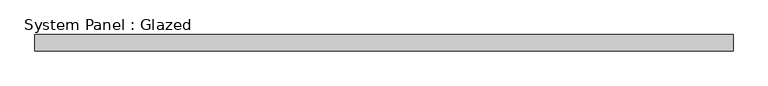
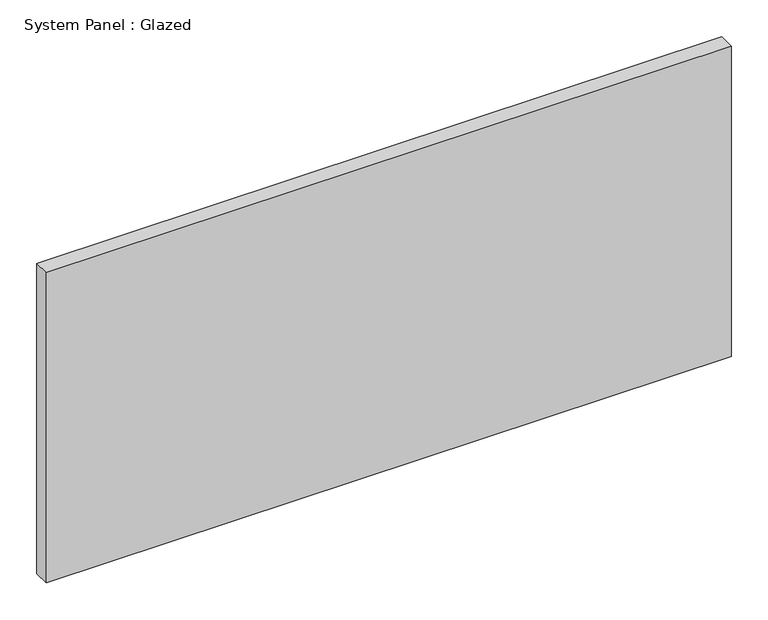
"""IFC4 building model written with IfcOpenShell, lengths in millimetres: plate geometry, System Panel : Glazed."""

from ifc_helpers import new_model, si_unit, origin, origin_with_axes, place, context, project, spatial, polyline, outline, extrude, source, transform, mapped, element, save


def system_panel_glazed_ed20128f(model_context):
    return source(origin(), model_context, "Body", "SweptSolid", [
        extrude(outline(polyline([(536.5750001, 19.05), (-536.5750001, 19.05), (-536.5750001, 44.45), (536.5750001, 44.45), (536.5750001, 19.05)])), origin_with_axes(), (0.0, 0.0, 1.0), 514.35),
    ])


if __name__ == "__main__":
    model = new_model("IFC4")
    model_context = context("Model", 3, world=origin())
    ifc_project = project(units=[si_unit("LENGTHUNIT", "METRE", prefix="MILLI")], contexts=[model_context])
    site = spatial("IfcSite", under=ifc_project)
    building = spatial("IfcBuilding", under=site)
    placement = place(None, origin())
    system_panel_glazed_shape = system_panel_glazed_ed20128f(model_context)
    element("IfcPlate", 1, ObjectType="System Panel : Glazed", at=placement, inside=building, context=model_context, shape_type="MappedRepresentation", body=[
        mapped(system_panel_glazed_shape, transform((0.0, 0.0, 0.0), x_axis=(1.0, 0.0, 0.0), y_axis=(0.0, 1.0, 0.0), z_axis=(0.0, 0.0, 1.0))),
    ])
    save(model, "model.ifc")

# Revit data of these elements
# Type "System Panel : Glazed"
#   Construction Type Id = "GSP4R"
#   Analytic Construction = "1/8 in Pilkington single glazing"
#   Visual Light Transmittance = 0.9
#   Solar Heat Gain Coefficient = 0.86
#   Heat Transfer Coefficient (U) = 1.18115 BTU/(h·ft²·°F)
#   Define Thermal Properties by = 1
# Element 1 (IfcPlate, "System Panel : Glazed")
#   Materials on its faces: "glass panel 223"
# Materials
#   "glass panel 223": class "Generic", colour RGB 120 120 120, transparency 0, Cost = 0
